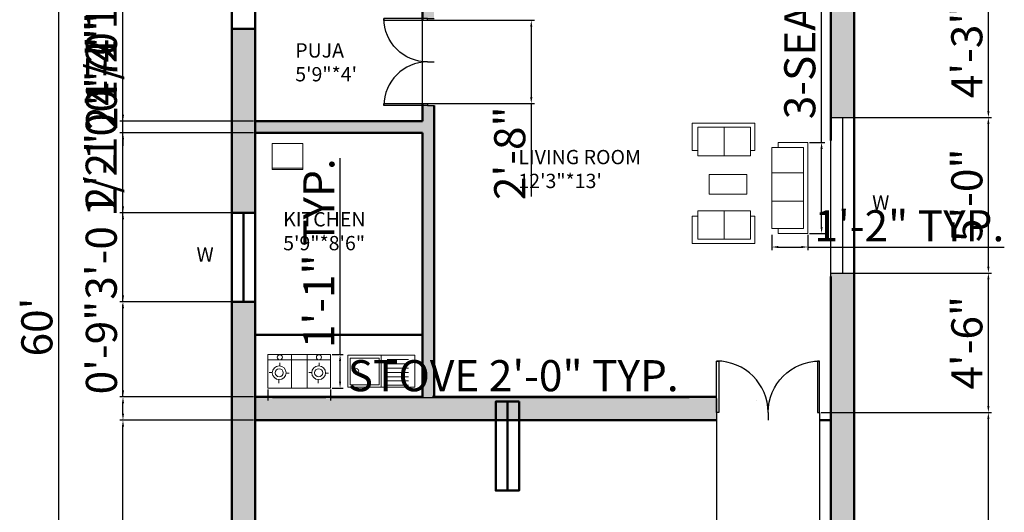
# Model space of a CAD drawing. Units: inches. Extents: x 2063 to 3370, y 2091 to 2971.
# Tile 12 of 14: x 2986 to 3365, y 2433 to 2623. Entities that reach past the tile are written whole.
import ezdxf

# ---------------------------------------------------------------- set-up
doc = ezdxf.new("R2010")
doc.units = ezdxf.units.IN
for name, color, linetype, lineweight in [('A-ANNO-DIMS', 2, 'Continuous', 18), ('A-ANNO-TEXT', 7, 'Continuous', 18), ('A-AREA-IDEN', 3, 'Continuous', 18), ('A-COLS', 7, 'Continuous', 50), ('A-DOOR', 4, 'Continuous', 25), ('A-EQPM', 8, 'Continuous', 18), ('A-FLOR-FIXT', 9, 'Continuous', 18), ('A-FURN', 8, 'Continuous', 18), ('A-GLAZ', 131, 'Continuous', 25), ('A-WALL', 7, 'Continuous', 50), ('A-WALL-PATT', 8, 'Continuous', 13)]:
    doc.layers.add(name, color=color, linetype=linetype, lineweight=lineweight)
doc.styles.get("Standard").update_dxf_attribs({"font": 'arial.ttf'})
doc.dimstyles.new('ISO-25', dxfattribs={"dimtxt": 12, "dimasz": 2.5, "dimexe": 1.25, "dimexo": 0.625, "dimtad": 1, "dimdec": 0, "dimlunit": 4, "dimtxsty": 'Standard', "dimcen": 2.5, "dimadec": 0, "dimazin": 0, "dimtfac": 1, "dimtdec": 0, "dimtmove": 0, "dimatfit": 3, "dimfxl": 1, "dimarcsym": 0})

# ---------------------------------------------------------------- blocks, each defined once
blk = doc.blocks.new('*D10')
at = {"layer": 'A-ANNO-DIMS', "color": 0, "lineweight": -2, "transparency": 16777216}
for p, q in [((3066.79, 2864.43), (2999.25, 2864.43)), ((3000.5, 2861.93), (3000.5, 2146.93)), ((3066.79, 2144.43), (2999.25, 2144.43))]:
    blk.add_line(p, q, dxfattribs=at)
at = {"layer": 'A-ANNO-DIMS', "color": 0, "transparency": 16777216}
for points in [[(3000.09, 2861.93), (3000.92, 2861.93), (3000.5, 2864.43)], [(3000.09, 2146.93), (3000.92, 2146.93), (3000.5, 2144.43)]]:
    blk.add_solid(points, dxfattribs=at)
at = {"layer": 'Defpoints', "color": 0, "transparency": 16777216}
for p in [(3067.42, 2864.43), (3000.5, 2144.43), (3067.42, 2144.43)]:
    blk.add_point(p, dxfattribs=at)
at = {"layer": 'A-ANNO-DIMS', "color": 0, "transparency": 16777216, "insert": (2993.75, 2504.43), "char_height": 12, "attachment_point": 5, "rotation": 90}
blk.add_mtext("60'", dxfattribs=at)
blk = doc.blocks.new('*U2')
for p, q in [((0, 0), (0, -6)), ((40, 0), (40, -6))]:
    blk.add_line(p, q)
blk.add_lwpolyline([(0, 0), (0, 40), (1.75, 40), (1.75, 0)], close=True)
blk.add_arc((0, 0), 40, 0, 90)
blk = doc.blocks.new('SOFA-2SEAT')
for p, q in [((0, 2.07), (0, 12.63)), ((0, 12.63), (24.16, 12.63)), ((24.16, 12.63), (24.16, 2.07)), ((12.27, 11.03), (12.27, 0)), ((2.08, 2.07), (0, 2.07)), ((24.16, 2.07), (22.46, 2.07))]:
    blk.add_line(p, q)
blk.add_lwpolyline([(22.46, 0), (2.08, 0), (2.08, 11.03), (22.46, 11.03)], close=True)
blk = doc.blocks.new('SOFA-3SEAT')
for p, q in [((2.4, 33.13), (2.4, 35.12)), ((2.4, 35.12), (13.91, 35.12)), ((13.91, 35.12), (13.91, 0)), ((0, 23.31), (12.18, 23.31)), ((0, 12.42), (12.18, 12.42)), ((2.4, 0), (2.4, 1.81)), ((13.91, 0), (2.4, 0))]:
    blk.add_line(p, q)
blk.add_lwpolyline([(12.18, 33.13), (0, 33.13), (0, 1.81), (12.18, 1.81)], close=True)
blk = doc.blocks.new('SINK')
for p, q in [((12.88, 12.38), (12.88, 0)), ((15.15, 10.72), (23.41, 10.72)), ((15.15, 9.06), (23.41, 9.06)), ((15.15, 7.39), (23.41, 7.39)), ((15.15, 5.73), (23.41, 5.73)), ((15.15, 4.07), (23.41, 4.07)), ((15.15, 2.41), (23.41, 2.41)), ((15.15, 0.75), (23.41, 0.75))]:
    blk.add_line(p, q)
for points in [[(25.76, 12.38), (0, 12.38), (0, 0), (25.76, 0)], [(0.92, 11.24), (12.1, 11.24), (12.1, 0.97), (0.92, 0.97)]]:
    blk.add_lwpolyline(points, close=True)
blk.add_circle((3.27, 6.25), 0.918)
blk = doc.blocks.new('STOVE')
for p, q in [((0, 12.93), (9.11, 12.93)), ((9.11, 12.93), (9.11, 0)), ((15.17, 0), (15.17, 12.93)), ((0, 10.85), (24.22, 10.85)), ((4.55, 8.54), (4.55, 9.68)), ((19.76, 8.54), (19.76, 9.68)), ((1.72, 5.99), (0.55, 5.99)), ((7.04, 5.79), (8.23, 5.79)), ((16.93, 5.99), (15.75, 5.99)), ((22.25, 5.79), (23.43, 5.79)), ((4.22, 3.16), (4.22, 1.87)), ((24.22, 0), (15.17, 0)), ((19.43, 3.16), (19.43, 1.87))]:
    blk.add_line(p, q)
blk.add_lwpolyline([(0, 12.93), (24.22, 12.93), (24.22, 0), (0, 0)], close=True)
for centre, radius in [((4.62, 11.87), 0.973), ((19.71, 11.87), 0.973), ((4.38, 5.88), 2.66), ((19.59, 5.88), 2.66), ((4.38, 5.88), 1.57), ((19.59, 5.88), 1.57)]:
    blk.add_circle(centre, radius)
blk = doc.blocks.new('*D26')
at = {"layer": 'A-ANNO-DIMS', "color": 0, "lineweight": -2, "transparency": 16777216}
for p, q in [((3294.89, 2575.71), (3294.89, 2775.57)), ((3290.25, 2575.71), (3296.14, 2575.71)), ((3294.89, 2543.09), (3294.89, 2573.21)), ((3290.25, 2540.59), (3296.14, 2540.59))]:
    blk.add_line(p, q, dxfattribs=at)
at = {"layer": 'A-ANNO-DIMS', "color": 0, "transparency": 16777216}
for points in [[(3294.47, 2573.21), (3295.31, 2573.21), (3294.89, 2575.71)], [(3294.47, 2543.09), (3295.31, 2543.09), (3294.89, 2540.59)]]:
    blk.add_solid(points, dxfattribs=at)
at = {"layer": 'Defpoints', "color": 0, "transparency": 16777216}
for p in [(3289.62, 2575.71), (3294.89, 2575.71), (3289.62, 2540.59)]:
    blk.add_point(p, dxfattribs=at)
at = {"layer": 'A-ANNO-DIMS', "color": 0, "transparency": 16777216, "insert": (3288.05, 2676.89), "char_height": 12, "attachment_point": 5, "rotation": 90}
blk.add_mtext('3-SEAT SOFA 2\'-11" TYP.', dxfattribs=at)
blk = doc.blocks.new('*D27')
at = {"layer": 'A-ANNO-DIMS', "color": 0, "lineweight": -2, "transparency": 16777216}
for p, q in [((3275.71, 2539.96), (3275.71, 2534.07)), ((3289.62, 2539.96), (3289.62, 2534.07)), ((3278.21, 2535.32), (3287.12, 2535.32)), ((3289.62, 2535.32), (3365.39, 2535.32))]:
    blk.add_line(p, q, dxfattribs=at)
at = {"layer": 'A-ANNO-DIMS', "color": 0, "transparency": 16777216}
for points in [[(3278.21, 2535.73), (3278.21, 2534.9), (3275.71, 2535.32)], [(3287.12, 2535.73), (3287.12, 2534.9), (3289.62, 2535.32)]]:
    blk.add_solid(points, dxfattribs=at)
at = {"layer": 'Defpoints', "color": 0, "transparency": 16777216}
for p in [(3275.71, 2540.59), (3289.62, 2540.59), (3289.62, 2535.32)]:
    blk.add_point(p, dxfattribs=at)
at = {"layer": 'A-ANNO-DIMS', "color": 0, "transparency": 16777216, "insert": (3328.76, 2541.97), "char_height": 12, "attachment_point": 5}
blk.add_mtext('1\'-2" TYP.', dxfattribs=at)
blk = doc.blocks.new('*D30')
at = {"layer": 'A-ANNO-DIMS', "color": 0, "lineweight": -2, "transparency": 16777216}
for p, q in [((3081.31, 2480.25), (3081.31, 2476)), ((3105.53, 2480.25), (3105.53, 2476)), ((3083.81, 2477.25), (3103.03, 2477.25)), ((3105.53, 2477.25), (3243.85, 2477.25))]:
    blk.add_line(p, q, dxfattribs=at)
at = {"layer": 'A-ANNO-DIMS', "color": 0, "transparency": 16777216}
for points in [[(3083.81, 2477.66), (3083.81, 2476.83), (3081.31, 2477.25)], [(3103.03, 2477.66), (3103.03, 2476.83), (3105.53, 2477.25)]]:
    blk.add_solid(points, dxfattribs=at)
at = {"layer": 'Defpoints', "color": 0, "transparency": 16777216}
for p in [(3081.31, 2480.88), (3105.53, 2480.88), (3105.53, 2477.25)]:
    blk.add_point(p, dxfattribs=at)
at = {"layer": 'A-ANNO-DIMS', "color": 0, "transparency": 16777216, "insert": (3175.94, 2484.08), "char_height": 12, "attachment_point": 5}
blk.add_mtext('STOVE 2\'-0" TYP.', dxfattribs=at)
blk = doc.blocks.new('*D31')
at = {"layer": 'A-ANNO-DIMS', "color": 0, "lineweight": -2, "transparency": 16777216}
for p, q in [((3109.16, 2493.81), (3109.16, 2569.57)), ((3106.15, 2493.81), (3110.41, 2493.81)), ((3109.16, 2483.38), (3109.16, 2491.31)), ((3106.15, 2480.88), (3110.41, 2480.88))]:
    blk.add_line(p, q, dxfattribs=at)
at = {"layer": 'A-ANNO-DIMS', "color": 0, "transparency": 16777216}
for points in [[(3108.74, 2491.31), (3109.58, 2491.31), (3109.16, 2493.81)], [(3108.74, 2483.38), (3109.58, 2483.38), (3109.16, 2480.88)]]:
    blk.add_solid(points, dxfattribs=at)
at = {"layer": 'Defpoints', "color": 0, "transparency": 16777216}
for p in [(3105.53, 2493.81), (3109.16, 2493.81), (3105.53, 2480.88)]:
    blk.add_point(p, dxfattribs=at)
at = {"layer": 'A-ANNO-DIMS', "color": 0, "transparency": 16777216, "insert": (3102.51, 2532.94), "char_height": 12, "attachment_point": 5, "rotation": 90}
blk.add_mtext('1\'-1" TYP.', dxfattribs=at)
blk = doc.blocks.new('*D148')
at = {"layer": 'A-ANNO-DIMS', "color": 0, "lineweight": -2, "transparency": 16777216}
for p, q in [((3076.42, 2584.55), (3076.42, 2907.68)), ((3078.92, 2906.43), (3138.42, 2906.43)), ((3140.92, 2584.55), (3140.92, 2907.68))]:
    blk.add_line(p, q, dxfattribs=at)
at = {"layer": 'A-ANNO-DIMS', "color": 0, "transparency": 16777216}
for points in [[(3078.92, 2906.84), (3078.92, 2906.01), (3076.42, 2906.43)], [(3138.42, 2906.84), (3138.42, 2906.01), (3140.92, 2906.43)]]:
    blk.add_solid(points, dxfattribs=at)
at = {"layer": 'Defpoints', "color": 0, "transparency": 16777216}
for p in [(3140.92, 2906.43), (3076.42, 2583.93), (3140.92, 2583.93)]:
    blk.add_point(p, dxfattribs=at)
at = {"layer": 'A-ANNO-DIMS', "color": 0, "transparency": 16777216, "insert": (3108.67, 2913.26), "char_height": 12, "attachment_point": 5}
blk.add_mtext('5\'-4 1/2"', dxfattribs=at)
blk = doc.blocks.new('*D151')
at = {"layer": 'A-ANNO-DIMS', "color": 0, "lineweight": -2, "transparency": 16777216}
for p, q in [((3075.79, 2468.43), (3024.17, 2468.43)), ((3025.42, 2236.93), (3025.42, 2465.93)), ((3075.79, 2234.43), (3024.17, 2234.43))]:
    blk.add_line(p, q, dxfattribs=at)
at = {"layer": 'A-ANNO-DIMS', "color": 0, "transparency": 16777216}
for points in [[(3025, 2465.93), (3025.83, 2465.93), (3025.42, 2468.43)], [(3025, 2236.93), (3025.83, 2236.93), (3025.42, 2234.43)]]:
    blk.add_solid(points, dxfattribs=at)
at = {"layer": 'Defpoints', "color": 0, "transparency": 16777216}
for p in [(3025.42, 2468.43), (3076.42, 2468.43), (3076.42, 2234.43)]:
    blk.add_point(p, dxfattribs=at)
at = {"layer": 'A-ANNO-DIMS', "color": 0, "transparency": 16777216, "insert": (3018.66, 2351.43), "char_height": 12, "attachment_point": 5, "rotation": 90}
blk.add_mtext('19\'-6"', dxfattribs=at)
blk = doc.blocks.new('*D152')
at = {"layer": 'A-ANNO-DIMS', "color": 0, "lineweight": -2, "transparency": 16777216}
for p, q in [((3025.42, 2477.43), (3025.42, 2513.08)), ((3075.79, 2477.43), (3024.17, 2477.43)), ((3025.42, 2470.93), (3025.42, 2474.93)), ((3075.79, 2468.43), (3024.17, 2468.43))]:
    blk.add_line(p, q, dxfattribs=at)
at = {"layer": 'A-ANNO-DIMS', "color": 0, "transparency": 16777216}
for points in [[(3025, 2474.93), (3025.83, 2474.93), (3025.42, 2477.43)], [(3025, 2470.93), (3025.83, 2470.93), (3025.42, 2468.43)]]:
    blk.add_solid(points, dxfattribs=at)
at = {"layer": 'Defpoints', "color": 0, "transparency": 16777216}
for p in [(3025.42, 2477.43), (3076.42, 2477.43), (3076.42, 2468.43)]:
    blk.add_point(p, dxfattribs=at)
at = {"layer": 'A-ANNO-DIMS', "color": 0, "transparency": 16777216, "insert": (3018.66, 2496.5), "char_height": 12, "attachment_point": 5, "rotation": 90}
blk.add_mtext('0\'-9"', dxfattribs=at)
blk = doc.blocks.new('*D153')
at = {"layer": 'A-ANNO-DIMS', "color": 0, "lineweight": -2, "transparency": 16777216}
for p, q in [((3025.42, 2514.15), (3025.42, 2577.75)), ((3075.79, 2514.15), (3024.17, 2514.15)), ((3025.42, 2479.93), (3025.42, 2511.65)), ((3075.79, 2477.43), (3024.17, 2477.43))]:
    blk.add_line(p, q, dxfattribs=at)
at = {"layer": 'A-ANNO-DIMS', "color": 0, "transparency": 16777216}
for points in [[(3025, 2511.65), (3025.83, 2511.65), (3025.42, 2514.15)], [(3025, 2479.93), (3025.83, 2479.93), (3025.42, 2477.43)]]:
    blk.add_solid(points, dxfattribs=at)
at = {"layer": 'Defpoints', "color": 0, "transparency": 16777216}
for p in [(3025.42, 2514.15), (3076.42, 2514.15), (3076.42, 2477.43)]:
    blk.add_point(p, dxfattribs=at)
at = {"layer": 'A-ANNO-DIMS', "color": 0, "transparency": 16777216, "insert": (3018.58, 2547.2), "char_height": 12, "attachment_point": 5, "rotation": 90}
blk.add_mtext('3\'-0 1/2"', dxfattribs=at)
blk = doc.blocks.new('*D154')
at = {"layer": 'A-ANNO-DIMS', "color": 0, "lineweight": -2, "transparency": 16777216}
for p, q in [((3025.42, 2548.5), (3025.42, 2621.64)), ((3075.79, 2548.5), (3024.17, 2548.5)), ((3025.42, 2516.65), (3025.42, 2546)), ((3075.79, 2514.15), (3024.17, 2514.15))]:
    blk.add_line(p, q, dxfattribs=at)
at = {"layer": 'A-ANNO-DIMS', "color": 0, "transparency": 16777216}
for points in [[(3025, 2546), (3025.83, 2546), (3025.42, 2548.5)], [(3025, 2516.65), (3025.83, 2516.65), (3025.42, 2514.15)]]:
    blk.add_solid(points, dxfattribs=at)
at = {"layer": 'Defpoints', "color": 0, "transparency": 16777216}
for p in [(3025.42, 2548.5), (3076.42, 2548.5), (3076.42, 2514.15)]:
    blk.add_point(p, dxfattribs=at)
at = {"layer": 'A-ANNO-DIMS', "color": 0, "transparency": 16777216, "insert": (3018.59, 2586.32), "char_height": 12, "attachment_point": 5, "rotation": 90}
blk.add_mtext('2\'-10 1/2"', dxfattribs=at)
blk = doc.blocks.new('*D155')
at = {"layer": 'A-ANNO-DIMS', "color": 0, "lineweight": -2, "transparency": 16777216}
for p, q in [((3025.42, 2579.43), (3025.42, 2615.28)), ((3075.79, 2579.43), (3024.17, 2579.43)), ((3025.42, 2551), (3025.42, 2576.93)), ((3075.79, 2548.5), (3024.17, 2548.5))]:
    blk.add_line(p, q, dxfattribs=at)
at = {"layer": 'A-ANNO-DIMS', "color": 0, "transparency": 16777216}
for points in [[(3025, 2576.93), (3025.83, 2576.93), (3025.42, 2579.43)], [(3025, 2551), (3025.83, 2551), (3025.42, 2548.5)]]:
    blk.add_solid(points, dxfattribs=at)
at = {"layer": 'Defpoints', "color": 0, "transparency": 16777216}
for p in [(3025.42, 2579.43), (3076.42, 2579.43), (3076.42, 2548.5)]:
    blk.add_point(p, dxfattribs=at)
at = {"layer": 'A-ANNO-DIMS', "color": 0, "transparency": 16777216, "insert": (3018.77, 2598.6), "char_height": 12, "attachment_point": 5, "rotation": 90}
blk.add_mtext('2\'-7"', dxfattribs=at)
blk = doc.blocks.new('*D156')
at = {"layer": 'A-ANNO-DIMS', "color": 0, "lineweight": -2, "transparency": 16777216}
for p, q in [((3025.42, 2586.43), (3025.42, 2650.04)), ((3075.79, 2583.93), (3024.17, 2583.93)), ((3025.42, 2579.43), (3025.42, 2583.93)), ((3075.79, 2579.43), (3024.17, 2579.43)), ((3025.42, 2576.93), (3025.42, 2574.43))]:
    blk.add_line(p, q, dxfattribs=at)
at = {"layer": 'A-ANNO-DIMS', "color": 0, "transparency": 16777216}
for points in [[(3025, 2586.43), (3025.83, 2586.43), (3025.42, 2583.93)], [(3025, 2576.93), (3025.83, 2576.93), (3025.42, 2579.43)]]:
    blk.add_solid(points, dxfattribs=at)
at = {"layer": 'Defpoints', "color": 0, "transparency": 16777216}
for p in [(3025.42, 2583.93), (3076.42, 2583.93), (3076.42, 2579.43)]:
    blk.add_point(p, dxfattribs=at)
at = {"layer": 'A-ANNO-DIMS', "color": 0, "transparency": 16777216, "insert": (3018.59, 2619.48), "char_height": 12, "attachment_point": 5, "rotation": 90}
blk.add_mtext('0\'-4 1/2"', dxfattribs=at)
blk = doc.blocks.new('*D157')
at = {"layer": 'A-ANNO-DIMS', "color": 0, "lineweight": -2, "transparency": 16777216}
for p, q in [((3075.79, 2631.93), (3024.17, 2631.93)), ((3025.42, 2586.43), (3025.42, 2629.43)), ((3075.79, 2583.93), (3024.17, 2583.93))]:
    blk.add_line(p, q, dxfattribs=at)
at = {"layer": 'A-ANNO-DIMS', "color": 0, "transparency": 16777216}
for points in [[(3025, 2629.43), (3025.83, 2629.43), (3025.42, 2631.93)], [(3025, 2586.43), (3025.83, 2586.43), (3025.42, 2583.93)]]:
    blk.add_solid(points, dxfattribs=at)
at = {"layer": 'Defpoints', "color": 0, "transparency": 16777216}
for p in [(3025.42, 2631.93), (3076.42, 2631.93), (3076.42, 2583.93)]:
    blk.add_point(p, dxfattribs=at)
at = {"layer": 'A-ANNO-DIMS', "color": 0, "transparency": 16777216, "insert": (3018.66, 2607.93), "char_height": 12, "attachment_point": 5, "rotation": 90}
blk.add_mtext('4\'-0"', dxfattribs=at)
blk = doc.blocks.new('*D161')
at = {"layer": 'A-ANNO-DIMS', "color": 0, "lineweight": -2, "transparency": 16777216}
for p, q in [((3294.79, 2471.41), (3360.49, 2471.41)), ((3359.24, 2155.93), (3359.24, 2468.91)), ((3299.04, 2153.43), (3360.49, 2153.43))]:
    blk.add_line(p, q, dxfattribs=at)
at = {"layer": 'A-ANNO-DIMS', "color": 0, "transparency": 16777216}
for points in [[(3358.82, 2468.91), (3359.66, 2468.91), (3359.24, 2471.41)], [(3358.82, 2155.93), (3359.66, 2155.93), (3359.24, 2153.43)]]:
    blk.add_solid(points, dxfattribs=at)
at = {"layer": 'Defpoints', "color": 0, "transparency": 16777216}
for p in [(3294.16, 2471.41), (3359.24, 2471.41), (3298.42, 2153.43)]:
    blk.add_point(p, dxfattribs=at)
at = {"layer": 'A-ANNO-DIMS', "color": 0, "transparency": 16777216, "insert": (3352.49, 2312.42), "char_height": 12, "attachment_point": 5, "rotation": 90}
blk.add_mtext('26\'-6"', dxfattribs=at)
blk = doc.blocks.new('*D162')
at = {"layer": 'A-ANNO-DIMS', "color": 0, "lineweight": -2, "transparency": 16777216}
for p, q in [((3299.04, 2525.28), (3360.49, 2525.28)), ((3359.24, 2473.91), (3359.24, 2522.78)), ((3294.79, 2471.41), (3360.49, 2471.41))]:
    blk.add_line(p, q, dxfattribs=at)
at = {"layer": 'A-ANNO-DIMS', "color": 0, "transparency": 16777216}
for points in [[(3358.82, 2522.78), (3359.66, 2522.78), (3359.24, 2525.28)], [(3358.82, 2473.91), (3359.66, 2473.91), (3359.24, 2471.41)]]:
    blk.add_solid(points, dxfattribs=at)
at = {"layer": 'Defpoints', "color": 0, "transparency": 16777216}
for p in [(3298.42, 2525.28), (3359.24, 2525.28), (3294.16, 2471.41)]:
    blk.add_point(p, dxfattribs=at)
at = {"layer": 'A-ANNO-DIMS', "color": 0, "transparency": 16777216, "insert": (3352.49, 2498.34), "char_height": 12, "attachment_point": 5, "rotation": 90}
blk.add_mtext('4\'-6"', dxfattribs=at)
blk = doc.blocks.new('*D163')
at = {"layer": 'A-ANNO-DIMS', "color": 0, "lineweight": -2, "transparency": 16777216}
for p, q in [((3299.04, 2585.28), (3360.49, 2585.28)), ((3359.24, 2527.78), (3359.24, 2582.78)), ((3299.04, 2525.28), (3360.49, 2525.28))]:
    blk.add_line(p, q, dxfattribs=at)
at = {"layer": 'A-ANNO-DIMS', "color": 0, "transparency": 16777216}
for points in [[(3358.82, 2582.78), (3359.66, 2582.78), (3359.24, 2585.28)], [(3358.82, 2527.78), (3359.66, 2527.78), (3359.24, 2525.28)]]:
    blk.add_solid(points, dxfattribs=at)
at = {"layer": 'Defpoints', "color": 0, "transparency": 16777216}
for p in [(3298.42, 2585.28), (3359.24, 2585.28), (3298.42, 2525.28)]:
    blk.add_point(p, dxfattribs=at)
at = {"layer": 'A-ANNO-DIMS', "color": 0, "transparency": 16777216, "insert": (3352.49, 2555.28), "char_height": 12, "attachment_point": 5, "rotation": 90}
blk.add_mtext('5\'-0"', dxfattribs=at)
blk = doc.blocks.new('*D164')
at = {"layer": 'A-ANNO-DIMS', "color": 0, "lineweight": -2, "transparency": 16777216}
for p, q in [((3299.04, 2636.43), (3360.49, 2636.43)), ((3359.24, 2587.78), (3359.24, 2633.93)), ((3299.04, 2585.28), (3360.49, 2585.28))]:
    blk.add_line(p, q, dxfattribs=at)
at = {"layer": 'A-ANNO-DIMS', "color": 0, "transparency": 16777216}
for points in [[(3358.82, 2633.93), (3359.66, 2633.93), (3359.24, 2636.43)], [(3358.82, 2587.78), (3359.66, 2587.78), (3359.24, 2585.28)]]:
    blk.add_solid(points, dxfattribs=at)
at = {"layer": 'Defpoints', "color": 0, "transparency": 16777216}
for p in [(3298.42, 2636.43), (3359.24, 2636.43), (3298.42, 2585.28)]:
    blk.add_point(p, dxfattribs=at)
at = {"layer": 'A-ANNO-DIMS', "color": 0, "transparency": 16777216, "insert": (3352.48, 2610.85), "char_height": 12, "attachment_point": 5, "rotation": 90}
blk.add_mtext('4\'-3"', dxfattribs=at)
blk = doc.blocks.new('*D175')
at = {"layer": 'A-ANNO-DIMS', "color": 0, "lineweight": -2, "transparency": 16777216}
for p, q in [((3141.54, 2622.85), (3184.17, 2622.85)), ((3182.92, 2620.35), (3182.92, 2593.19)), ((3141.54, 2590.69), (3184.17, 2590.69)), ((3182.92, 2590.69), (3182.92, 2554.84))]:
    blk.add_line(p, q, dxfattribs=at)
at = {"layer": 'A-ANNO-DIMS', "color": 0, "transparency": 16777216}
for points in [[(3182.5, 2620.35), (3183.33, 2620.35), (3182.92, 2622.85)], [(3182.5, 2593.19), (3183.33, 2593.19), (3182.92, 2590.69)]]:
    blk.add_solid(points, dxfattribs=at)
at = {"layer": 'Defpoints', "color": 0, "transparency": 16777216}
for p in [(3140.92, 2622.85), (3140.92, 2590.69), (3182.92, 2590.69)]:
    blk.add_point(p, dxfattribs=at)
at = {"layer": 'A-ANNO-DIMS', "color": 0, "transparency": 16777216, "insert": (3176.16, 2571.52), "char_height": 12, "attachment_point": 5, "rotation": 90}
blk.add_mtext('2\'-8"', dxfattribs=at)
blk = doc.blocks.new('*D176')
at = {"layer": 'A-ANNO-DIMS', "color": 0, "lineweight": -2, "transparency": 16777216}
for p, q in [((3254.4, 2476.8), (3254.4, 2101.18)), ((3294.16, 2470.78), (3294.16, 2101.18)), ((3256.9, 2102.43), (3291.66, 2102.43))]:
    blk.add_line(p, q, dxfattribs=at)
at = {"layer": 'A-ANNO-DIMS', "color": 0, "transparency": 16777216}
for points in [[(3256.9, 2102.84), (3256.9, 2102.01), (3254.4, 2102.43)], [(3291.66, 2102.84), (3291.66, 2102.01), (3294.16, 2102.43)]]:
    blk.add_solid(points, dxfattribs=at)
at = {"layer": 'Defpoints', "color": 0, "transparency": 16777216}
for p in [(3254.4, 2477.43), (3294.16, 2471.41), (3294.16, 2102.43)]:
    blk.add_point(p, dxfattribs=at)
at = {"layer": 'A-ANNO-DIMS', "color": 0, "transparency": 16777216, "insert": (3274.28, 2109.18), "char_height": 12, "attachment_point": 5}
blk.add_mtext('3\'-4"', dxfattribs=at)

msp = doc.modelspace()

# ---------------------------------------------------------------- hatches: boundary and pattern name
at = {"layer": 'A-WALL-PATT'}
h = msp.add_hatch(color=256, dxfattribs=at)
h.dxf.hatch_style = 1
h.paths.add_polyline_path([(3181.8, 2234.43), (3076.42, 2234.43), (3076.42, 2232.93), (3076.42, 2225.43), (3181.8, 2225.43)])
h.paths.add_polyline_path([(3212.92, 2192.43), (3200.92, 2192.43), (3104.92, 2192.43), (3104.92, 2189.43), (3104.92, 2187.43), (3200.92, 2187.43), (3212.92, 2187.42)], flags=17)
h.paths.add_polyline_path([(3219.45, 2153.43), (3076.42, 2153.43), (3076.42, 2222.57), (3067.42, 2222.57), (3067.42, 2144.43), (3219.45, 2144.43)])
h.paths.add_polyline_path([(3076.42, 2343.93), (3076.42, 2351.28), (3067.42, 2351.28), (3067.42, 2241.68), (3076.42, 2241.68), (3076.42, 2258.43)])
h.paths.add_polyline_path([(3175.73, 2554.94), (3230.21, 2554.94), (3230.21, 2575.54), (3175.73, 2575.54)], flags=9)
h.paths.add_polyline_path([(3085.27, 2530.92), (3121.9, 2530.92), (3121.9, 2551.53), (3085.27, 2551.53)], flags=9)
h.paths.add_polyline_path([(3089.9, 2596.23), (3114.49, 2596.23), (3114.49, 2616.83), (3089.9, 2616.83)], flags=9)
h.paths.add_polyline_path([(3260.79, 2797.55), (3297.86, 2797.55), (3297.86, 2808.94), (3260.79, 2808.94)], flags=9)
h.paths.add_polyline_path([(3113.05, 2696.74), (3189.97, 2696.74), (3189.97, 2717.35), (3113.05, 2717.35)], flags=9)
h.paths.add_polyline_path([(3226.64, 2835.24), (3234.55, 2835.24), (3234.55, 2846.62), (3226.64, 2846.62)], flags=9)
h.paths.add_polyline_path([(3140.56, 2833.68), (3150.6, 2833.68), (3150.6, 2845.06), (3140.56, 2845.06)], flags=9)
h.paths.add_polyline_path([(3193.53, 2795.64), (3230.6, 2795.64), (3230.6, 2807.02), (3193.53, 2807.02)], flags=9)
h.paths.add_polyline_path([(3225.05, 2726.09), (3287.83, 2726.09), (3287.83, 2746.7), (3225.05, 2746.7)], flags=9)
h = msp.add_hatch(color=256, dxfattribs=at)
h.dxf.hatch_style = 1
h.paths.add_polyline_path([(3294.05, 2153.43), (3219.45, 2153.43), (3219.45, 2144.43), (3294.05, 2144.43)])
h.paths.add_polyline_path([(3307.42, 2220.3), (3298.42, 2220.3), (3298.42, 2153.43), (3294.05, 2153.43), (3294.05, 2144.43), (3307.42, 2144.43)])
h.paths.add_polyline_path([(3076.42, 2468.43), (3076.42, 2477.43), (3076.42, 2514.15), (3067.42, 2514.15), (3067.42, 2370.39), (3076.42, 2370.39)])
h.paths.add_polyline_path([(3307.42, 2525.28), (3298.42, 2525.28), (3298.42, 2523.93), (3298.42, 2466.93), (3298.42, 2383.04), (3307.42, 2383.04)])
h.paths.add_polyline_path([(3307.42, 2363.93), (3298.42, 2363.93), (3298.42, 2239.41), (3307.42, 2239.41)])
h.paths.add_polyline_path([(3235.32, 2180.53), (3274.95, 2180.53), (3274.95, 2201.14), (3235.32, 2201.14)], flags=9)
h.paths.add_polyline_path([(3127.74, 2323.36), (3191.84, 2323.36), (3191.84, 2343.96), (3127.74, 2343.96)], flags=9)
h.paths.add_polyline_path([(3175.73, 2554.94), (3230.21, 2554.94), (3230.21, 2575.54), (3175.73, 2575.54)], flags=9)
h.paths.add_polyline_path([(3085.27, 2530.92), (3121.9, 2530.92), (3121.9, 2551.53), (3085.27, 2551.53)], flags=9)
h.paths.add_polyline_path([(3089.9, 2596.23), (3114.49, 2596.23), (3114.49, 2616.83), (3089.9, 2616.83)], flags=9)
h.paths.add_polyline_path([(3260.79, 2797.55), (3297.86, 2797.55), (3297.86, 2808.94), (3260.79, 2808.94)], flags=9)
h.paths.add_polyline_path([(3113.05, 2696.74), (3189.97, 2696.74), (3189.97, 2717.35), (3113.05, 2717.35)], flags=9)
h.paths.add_polyline_path([(3226.64, 2835.24), (3234.55, 2835.24), (3234.55, 2846.62), (3226.64, 2846.62)], flags=9)
h.paths.add_polyline_path([(3140.56, 2833.68), (3150.6, 2833.68), (3150.6, 2845.06), (3140.56, 2845.06)], flags=9)
h.paths.add_polyline_path([(3193.53, 2795.64), (3230.6, 2795.64), (3230.6, 2807.02), (3193.53, 2807.02)], flags=9)
h.paths.add_polyline_path([(3225.05, 2726.09), (3287.83, 2726.09), (3287.83, 2746.7), (3225.05, 2746.7)], flags=9)
h = msp.add_hatch(color=256, dxfattribs=at)
h.dxf.hatch_style = 1
h.paths.add_polyline_path([(3076.42, 2619.52), (3067.42, 2619.52), (3067.42, 2548.5), (3076.42, 2548.5), (3076.42, 2579.43)])
h.paths.add_polyline_path([(3236.69, 2636.43), (3197.92, 2636.43), (3197.92, 2631.93), (3236.69, 2631.93)])
h.paths.add_polyline_path([(3145.42, 2631.93), (3149.1, 2631.93), (3149.1, 2636.43), (3147.77, 2636.43), (3076.42, 2636.43), (3076.42, 2631.93), (3113.39, 2631.93), (3136.42, 2631.93), (3140.92, 2631.93), (3140.92, 2623.58), (3142.89, 2623.58), (3145.42, 2623.58)])
h.paths.add_polyline_path([(3298.42, 2636.43), (3276.69, 2636.43), (3276.69, 2631.93), (3298.42, 2631.93)])
h.paths.add_polyline_path([(3307.42, 2679.03), (3298.42, 2679.03), (3298.42, 2645.28), (3307.42, 2645.28)])
h.paths.add_polyline_path([(3307.42, 2626.16), (3298.42, 2626.16), (3298.42, 2585.28), (3307.42, 2585.28)])
h.paths.add_polyline_path([(3260.79, 2797.55), (3297.86, 2797.55), (3297.86, 2808.94), (3260.79, 2808.94)], flags=9)
h.paths.add_polyline_path([(3113.05, 2696.74), (3189.97, 2696.74), (3189.97, 2717.35), (3113.05, 2717.35)], flags=9)
h.paths.add_polyline_path([(3226.64, 2835.24), (3234.55, 2835.24), (3234.55, 2846.62), (3226.64, 2846.62)], flags=9)
h.paths.add_polyline_path([(3140.56, 2833.68), (3150.6, 2833.68), (3150.6, 2845.06), (3140.56, 2845.06)], flags=9)
h.paths.add_polyline_path([(3193.53, 2795.64), (3230.6, 2795.64), (3230.6, 2807.02), (3193.53, 2807.02)], flags=9)
h.paths.add_polyline_path([(3225.05, 2726.09), (3287.83, 2726.09), (3287.83, 2746.7), (3225.05, 2746.7)], flags=9)
h = msp.add_hatch(color=256, dxfattribs=at)
h.dxf.hatch_style = 1
h.paths.add_polyline_path([(3119.94, 2831.43), (3076.42, 2831.43), (3076.42, 2822.43), (3119.94, 2822.43)])
h.paths.add_polyline_path([(3186.73, 2831.43), (3167.94, 2831.43), (3167.94, 2822.43), (3186.73, 2822.43)])
h.paths.add_polyline_path([(3219.33, 2831.43), (3205.84, 2831.43), (3205.84, 2822.43), (3219.33, 2822.43)])
h.paths.add_polyline_path([(3298.42, 2831.43), (3243.76, 2831.43), (3243.76, 2822.43), (3298.42, 2822.43)])
h.paths.add_polyline_path([(3235.32, 2180.53), (3274.95, 2180.53), (3274.95, 2201.14), (3235.32, 2201.14)], flags=9)
h.paths.add_polyline_path([(3127.74, 2323.36), (3191.84, 2323.36), (3191.84, 2343.96), (3127.74, 2343.96)], flags=9)
h.paths.add_polyline_path([(3175.73, 2554.94), (3230.21, 2554.94), (3230.21, 2575.54), (3175.73, 2575.54)], flags=9)
h.paths.add_polyline_path([(3085.27, 2530.92), (3121.9, 2530.92), (3121.9, 2551.53), (3085.27, 2551.53)], flags=9)
h.paths.add_polyline_path([(3089.9, 2596.23), (3114.49, 2596.23), (3114.49, 2616.83), (3089.9, 2616.83)], flags=9)
h.paths.add_polyline_path([(3113.05, 2696.74), (3189.97, 2696.74), (3189.97, 2717.35), (3113.05, 2717.35)], flags=9)
h.paths.add_polyline_path([(3193.53, 2795.64), (3230.6, 2795.64), (3230.6, 2807.02), (3193.53, 2807.02)], flags=9)
h.paths.add_polyline_path([(3225.05, 2726.09), (3287.83, 2726.09), (3287.83, 2746.7), (3225.05, 2746.7)], flags=9)
h = msp.add_hatch(color=256, dxfattribs=at)
h.dxf.hatch_style = 1
h.paths.add_polyline_path([(3254.4, 2477.43), (3145.42, 2477.43), (3145.42, 2579.43), (3145.42, 2589.96), (3142.89, 2589.96), (3140.92, 2589.96), (3140.92, 2583.93), (3131.92, 2583.93), (3076.42, 2583.93), (3076.42, 2579.43), (3136.42, 2579.43), (3140.92, 2579.43), (3140.92, 2477.43), (3076.42, 2477.43), (3076.42, 2468.43), (3193.42, 2468.43), (3254.4, 2468.43), (3254.4, 2471.41)])
h.paths.add_polyline_path([(3235.32, 2180.53), (3274.95, 2180.53), (3274.95, 2201.14), (3235.32, 2201.14)], flags=9)
h.paths.add_polyline_path([(3127.74, 2323.36), (3191.84, 2323.36), (3191.84, 2343.96), (3127.74, 2343.96)], flags=9)
h.paths.add_polyline_path([(3175.73, 2554.94), (3230.21, 2554.94), (3230.21, 2575.54), (3175.73, 2575.54)], flags=25)
h.paths.add_polyline_path([(3089.9, 2596.23), (3114.49, 2596.23), (3114.49, 2616.83), (3089.9, 2616.83)], flags=9)
h.paths.add_polyline_path([(3260.79, 2797.55), (3297.86, 2797.55), (3297.86, 2808.94), (3260.79, 2808.94)], flags=9)
h.paths.add_polyline_path([(3113.05, 2696.74), (3189.97, 2696.74), (3189.97, 2717.35), (3113.05, 2717.35)], flags=9)
h.paths.add_polyline_path([(3193.53, 2795.64), (3230.6, 2795.64), (3230.6, 2807.02), (3193.53, 2807.02)], flags=9)
h.paths.add_polyline_path([(3225.05, 2726.09), (3287.83, 2726.09), (3287.83, 2746.7), (3225.05, 2746.7)], flags=9)

# ---------------------------------------------------------------- linework, layer by layer
at = {"layer": 'A-COLS'}
msp.add_lwpolyline([(3067.42, 2638.63), (3076.42, 2638.63), (3076.42, 2619.52), (3067.42, 2619.52)], close=True, dxfattribs=at)
at = {"layer": 'A-EQPM'}
msp.add_line((3083.02, 2565.71), (3094.83, 2565.71), dxfattribs=at)
msp.add_lwpolyline([(3083.02, 2575.31), (3094.83, 2575.31), (3094.83, 2565.19), (3083.02, 2565.19)], close=True, dxfattribs=at)
at = {"layer": 'A-FURN'}
msp.add_lwpolyline([(3251.57, 2563.33), (3266.05, 2563.33), (3266.05, 2555.77), (3251.57, 2555.77)], close=True, dxfattribs=at)
at = {"layer": 'A-GLAZ'}
for p, q in [((3298.42, 2528.28), (3298.42, 2585.28)), ((3298.42, 2585.28), (3307.42, 2585.28)), ((3302.92, 2585.28), (3302.92, 2525.28)), ((3298.42, 2525.28), (3307.42, 2525.28))]:
    msp.add_line(p, q, dxfattribs=at)
for points in [[(3298.42, 2532.78), (3298.42, 2580.78)], [(3298.42, 2523.93), (3298.42, 2571.93)]]:
    msp.add_lwpolyline(points, dxfattribs=at)
at = {"layer": 'A-WALL'}
for p, q in [((3140.92, 2622.85), (3140.92, 2631.93)), ((3140.92, 2583.93), (3140.92, 2590.69)), ((3145.42, 2579.43), (3145.42, 2589.96)), ((3076.42, 2583.93), (3136.42, 2583.93)), ((3131.92, 2583.93), (3140.92, 2583.93)), ((3076.42, 2579.43), (3136.42, 2579.43)), ((3076.42, 2579.43), (3076.42, 2477.43)), ((3140.92, 2579.43), (3131.95, 2579.43)), ((3140.92, 2477.43), (3140.92, 2579.43)), ((3145.42, 2477.43), (3145.42, 2579.43)), ((3071.92, 2548.5), (3071.92, 2514.15)), ((3298.42, 2466.93), (3298.42, 2523.93)), ((3076.42, 2477.43), (3076.47, 2501.43)), ((3076.47, 2501.43), (3140.92, 2501.43)), ((3076.42, 2477.43), (3140.92, 2477.43)), ((3076.42, 2477.43), (3140.92, 2477.43)), ((3076.42, 2241.68), (3076.42, 2477.43)), ((3144.81, 2477.43), (3197.31, 2477.43)), ((3145.42, 2477.43), (3254.4, 2477.43)), ((3197.31, 2477.43), (3249.81, 2477.43)), ((3173.74, 2475.64), (3173.74, 2441.3)), ((3269.94, 2476.04), (3269.94, 2476.04)), ((3076.42, 2468.43), (3145.42, 2468.43)), ((3076.42, 2468.43), (3193.42, 2468.43)), ((3076.42, 2468.43), (3076.42, 2348.43)), ((3145.42, 2468.43), (3254.4, 2468.43)), ((3197.31, 2468.43), (3245.31, 2468.43)), ((3294.16, 2468.43), (3298.42, 2468.43))]:
    msp.add_line(p, q, dxfattribs=at)
for points in [[(3067.42, 2144.43), (3307.42, 2144.43), (3307.42, 2864.43), (3067.42, 2864.43)], [(3076.42, 2548.5), (3067.42, 2548.5), (3067.42, 2514.15), (3076.42, 2514.15)], [(3178.24, 2475.64), (3169.24, 2475.64), (3169.24, 2441.3), (3178.24, 2441.3)]]:
    msp.add_lwpolyline(points, close=True, dxfattribs=at)
for points in [[(3076.42, 2822.43), (3076.42, 2576.43)], [(3298.42, 2576.43), (3298.42, 2769.93)], [(3076.42, 2631.93), (3076.42, 2583.93)], [(3076.42, 2579.43), (3076.42, 2531.43)], [(3298.42, 2471.43), (3298.42, 2519.43)], [(3298.42, 2382.93), (3298.42, 2466.93)]]:
    msp.add_lwpolyline(points, dxfattribs=at)

# ---------------------------------------------------------------- block references
at = {"layer": 'A-DOOR', "yscale": 0.4203428619043682, "zscale": 0.4203428619043682, "rotation": 90}
for p, xscale in [((3142.89, 2623.58), -0.4203428619043682), ((3142.89, 2589.96), 0.4203428619043682)]:
    msp.add_blockref('*U2', p, dxfattribs=dict(at, xscale=xscale))
at = {"layer": 'A-DOOR', "yscale": 0.4970278449321303, "zscale": 0.4970278449321303}
for p, xscale in [((3254.4, 2471.41), 0.4970278449321303), ((3294.16, 2471.41), -0.4970278449321303)]:
    msp.add_blockref('*U2', p, dxfattribs=dict(at, xscale=xscale))
at = {"layer": 'A-FLOR-FIXT'}
for name, p in [('STOVE', (3081.31, 2480.88)), ('SINK', (3112.19, 2481.18))]:
    msp.add_blockref(name, p, dxfattribs=at)
at = {"layer": 'A-FURN'}
for name, p in [('SOFA-2SEAT', (3245.04, 2570.52)), ('SOFA-3SEAT', (3275.71, 2540.59))]:
    msp.add_blockref(name, p, dxfattribs=at)
at = {"layer": 'A-FURN', "extrusion": (0, 0, -1), "zscale": -1, "rotation": 180}
msp.add_blockref('SOFA-2SEAT', (-3245.04, 2549.32), dxfattribs=at)

# ---------------------------------------------------------------- texts
at = {"layer": 'A-ANNO-TEXT', "char_height": 5.52, "attachment_point": 1}
for insert in [(3314.42, 2555.25), (3053.79, 2535.17)]:
    msp.add_mtext_dynamic_manual_height_columns('W', width=106.0361, gutter_width=27.61, heights=[0], dxfattribs=dict(at, insert=insert))
at = {"layer": 'A-AREA-IDEN', "attachment_point": 1}
for s, heights, insert, char_height in [('PUJA \\P5\'9"*4\'', [14.84], (3091.87, 2613.99), 5.523), ('LIVING ROOM\\P12\'3"*13\'', [0], (3177.95, 2572.8), 5.5229), ('KITCHEN\\P5\'9"*8\'6"', [0], (3087.22, 2548.78), 5.523)]:
    msp.add_mtext_dynamic_manual_height_columns(s, width=106.0361, gutter_width=27.61, heights=heights, dxfattribs=dict(at, insert=insert, char_height=char_height))

# ---------------------------------------------------------------- dimensions: what is measured, and where the dimension line sits
at = {"layer": 'A-ANNO-DIMS'}
for base, p1, p2, picture, middle in [((3140.92, 2906.43), (3076.42, 2583.93), (3140.92, 2583.93), '*D148', (3108.67, 2913.26)), ((3294.16, 2102.43), (3254.4, 2477.43), (3294.16, 2471.41), '*D176', (3274.28, 2109.18))]:
    dim = msp.add_linear_dim(base=base, p1=p1, p2=p2, dimstyle='ISO-25', override={"dimdec": 1, "dimlfac": 1, "dimrnd": 0, "dimzin": 1, "dimdsep": 46, "dimlunit": 4, "dimfrac": 2}, dxfattribs=at)
    dim.commit()
    dim.dimension.update_dxf_attribs({"geometry": picture, "text_midpoint": middle})
for base, p1, p2, angle, override, picture, middle in [((3000.5, 2144.43), (3067.42, 2864.43), (3067.42, 2144.43), 90, {"dimclrd": 0, "dimclre": 0, "dimclrt": 0}, '*D10', (2993.75, 2504.43)), ((3025.42, 2583.93), (3076.42, 2579.43), (3076.42, 2583.93), 90, {"dimdec": 1, "dimlfac": 1, "dimrnd": 0, "dimzin": 1, "dimdsep": 46, "dimlunit": 4, "dimfrac": 2}, '*D156', (3018.59, 2619.48)), ((3359.2401, 2636.4264), (3298.4159, 2585.2786), (3298.4159, 2636.4264), 90, {"dimdec": 1, "dimlfac": 1, "dimrnd": 0, "dimzin": 1, "dimdsep": 46, "dimlunit": 4, "dimfrac": 2}, '*D164', (3352.4841, 2610.8525)), ((3025.42, 2631.93), (3076.42, 2583.93), (3076.42, 2631.93), 90, {"dimdec": 1, "dimlfac": 1, "dimrnd": 0, "dimzin": 1, "dimdsep": 46, "dimlunit": 4, "dimfrac": 2}, '*D157', (3018.66, 2607.93)), ((3025.4159, 2548.4974), (3076.4159, 2514.1508), (3076.4159, 2548.4974), 90, {"dimdec": 1, "dimlfac": 1, "dimrnd": 0, "dimzin": 1, "dimdsep": 46, "dimlunit": 4, "dimfrac": 2}, '*D154', (3018.5863, 2586.3168)), ((3182.92, 2590.69), (3140.92, 2622.85), (3140.92, 2590.69), 270, {"dimdec": 1, "dimlfac": 1, "dimrnd": 0, "dimzin": 1, "dimdsep": 46, "dimlunit": 4, "dimfrac": 2}, '*D175', (3176.16, 2571.52)), ((3025.42, 2579.43), (3076.42, 2548.5), (3076.42, 2579.43), 90, {"dimdec": 1, "dimlfac": 1, "dimrnd": 0, "dimzin": 1, "dimdsep": 46, "dimlunit": 4, "dimfrac": 2}, '*D155', (3018.77, 2598.6)), ((3359.24, 2585.28), (3298.42, 2525.28), (3298.42, 2585.28), 90, {"dimdec": 1, "dimlfac": 1, "dimrnd": 0, "dimzin": 1, "dimdsep": 46, "dimlunit": 4, "dimfrac": 2}, '*D163', (3352.49, 2555.28)), ((3025.42, 2514.15), (3076.42, 2477.43), (3076.42, 2514.15), 90, {"dimdec": 1, "dimlfac": 1, "dimrnd": 0, "dimzin": 1, "dimdsep": 46, "dimlunit": 4, "dimfrac": 2}, '*D153', (3018.58, 2547.2)), ((3359.24, 2525.28), (3294.16, 2471.41), (3298.42, 2525.28), 90, {"dimdec": 1, "dimlfac": 1, "dimrnd": 0, "dimzin": 1, "dimdsep": 46, "dimlunit": 4, "dimfrac": 2}, '*D162', (3352.49, 2498.34)), ((3025.42, 2477.43), (3076.42, 2468.43), (3076.42, 2477.43), 90, {"dimdec": 1, "dimlfac": 1, "dimrnd": 0, "dimzin": 1, "dimdsep": 46, "dimlunit": 4, "dimfrac": 2}, '*D152', (3018.66, 2496.5)), ((3359.24, 2471.41), (3298.42, 2153.43), (3294.16, 2471.41), 90, {"dimdec": 1, "dimlfac": 1, "dimrnd": 0, "dimzin": 1, "dimdsep": 46, "dimlunit": 4, "dimfrac": 2}, '*D161', (3352.49, 2312.42)), ((3025.42, 2468.43), (3076.42, 2234.43), (3076.42, 2468.43), 90, {"dimdec": 1, "dimlfac": 1, "dimrnd": 0, "dimzin": 1, "dimdsep": 46, "dimlunit": 4, "dimfrac": 2}, '*D151', (3018.66, 2351.43))]:
    dim = msp.add_linear_dim(base=base, p1=p1, p2=p2, angle=angle, dimstyle='ISO-25', override=override, dxfattribs=at)
    dim.commit()
    dim.dimension.update_dxf_attribs({"geometry": picture, "text_midpoint": middle})
for base, p1, p2, text, picture, middle in [((3294.89, 2575.71), (3289.62, 2540.59), (3289.62, 2575.71), '3-SEAT SOFA <> TYP.', '*D26', (3288.05, 2676.89)), ((3109.16, 2493.81), (3105.53, 2480.88), (3105.53, 2493.81), '<> TYP.', '*D31', (3102.51, 2532.94))]:
    dim = msp.add_linear_dim(base=base, p1=p1, p2=p2, angle=90, text=text, dimstyle='ISO-25', override={"dimdec": 1, "dimrnd": 0, "dimzin": 1, "dimlunit": 4, "dimfrac": 2}, dxfattribs=at)
    dim.commit()
    dim.dimension.update_dxf_attribs({"geometry": picture, "text_midpoint": middle})
for base, p1, p2, text, picture, middle in [((3289.62, 2535.32), (3275.71, 2540.59), (3289.62, 2540.59), '<> TYP.', '*D27', (3328.76, 2541.97)), ((3105.53, 2477.25), (3081.31, 2480.88), (3105.53, 2480.88), 'STOVE <> TYP.', '*D30', (3175.94, 2484.08))]:
    dim = msp.add_linear_dim(base=base, p1=p1, p2=p2, text=text, dimstyle='ISO-25', override={"dimdec": 1, "dimrnd": 0, "dimzin": 1, "dimlunit": 4, "dimfrac": 2}, dxfattribs=at)
    dim.commit()
    dim.dimension.update_dxf_attribs({"geometry": picture, "text_midpoint": middle})

doc.saveas('drawing.dxf')
